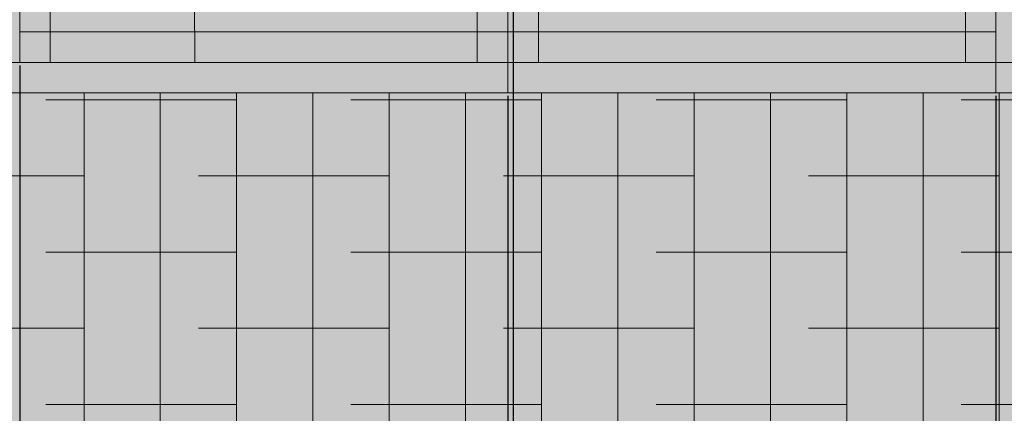
# Model space of a CAD drawing. Units: millimetres. Extents: x 11032 to 26788, y 3406 to 24505.
# Tile 13 of 78: x 17145 to 18758, y 6736 to 7381. Entities that reach past the tile are written whole.
import ezdxf

# ---------------------------------------------------------------- set-up
doc = ezdxf.new("R2010")
doc.units = ezdxf.units.MM
doc.header["$MEASUREMENT"] = 0
for name, color, linetype, lineweight in [('A-ANNO-DIMS', 2, 'Continuous', 18), ('A-GLAZ', 250, 'Continuous', 20), ('A-WALL-INTR', 8, 'Continuous', 18), ('A-WALL-PLIN-PATT', 253, 'Continuous', 13)]:
    doc.layers.add(name, color=color, linetype=linetype, lineweight=lineweight)
doc.layers.add('A-GLAZ-FRAM-PATT', color=250, linetype='Continuous', lineweight=13, true_color=0x262627)
doc.layers.add('A-WALL-INTR-PATT', color=251, linetype='Continuous', lineweight=13, true_color=0x6c6b6a)
doc.styles.get("Standard").update_dxf_attribs({"font": 'arial.ttf'})
doc.dimstyles.get("Standard").update_dxf_attribs({"dimtxt": 150, "dimasz": 100, "dimexe": 10, "dimexo": 5, "dimgap": 5, "dimtad": 0, "dimtih": 1, "dimtoh": 1, "dimdec": 0, "dimzin": 0, "dimdsep": 46, "dimtxsty": 'Standard', "dimcen": 0.09, "dimadec": 0, "dimazin": 0, "dimtfac": 1, "dimtdec": 0, "dimtofl": 0, "dimtmove": 0, "dimatfit": 3, "dimfxl": 1, "dimtolj": 1, "dimtzin": 0, "dimarcsym": 0})

# ---------------------------------------------------------------- blocks, each defined once
blk = doc.blocks.new('*D36')
at = {"layer": 'A-ANNO-DIMS', "color": 0, "lineweight": -2, "transparency": 16777216}
for p, q in [((12301.3, 17115.9), (12301.3, 24416.9)), ((25397.4, 4466.4), (25397.4, 24416.9)), ((12401.3, 24406.9), (18569.2, 24406.9)), ((25297.4, 24406.9), (19129.5, 24406.9))]:
    blk.add_line(p, q, dxfattribs=at)
at = {"layer": 'A-ANNO-DIMS', "color": 0, "transparency": 16777216}
for points in [[(12401.3, 24423.5), (12401.3, 24390.2), (12301.3, 24406.9)], [(25297.4, 24423.5), (25297.4, 24390.2), (25397.4, 24406.9)]]:
    blk.add_solid(points, dxfattribs=at)
at = {"layer": 'Defpoints', "color": 0, "transparency": 16777216}
for p in [(25397.4, 24406.9), (12301.3, 17110.9), (25397.4, 4461.4)]:
    blk.add_point(p, dxfattribs=at)
at = {"layer": 'A-ANNO-DIMS', "color": 0, "transparency": 16777216, "insert": (18849.3, 24406.9), "char_height": 150, "attachment_point": 5}
blk.add_mtext('\\A1;13096', dxfattribs=at)
blk = doc.blocks.new('*D37')
at = {"layer": 'A-ANNO-DIMS', "color": 0, "lineweight": -2, "transparency": 16777216}
for p, q in [((18087.7, 23450.4), (11334.8, 23450.4)), ((11344.8, 23350.4), (11344.8, 14037.5)), ((11344.8, 4561.4), (11344.8, 13874.3)), ((12927.7, 4461.4), (11334.8, 4461.4))]:
    blk.add_line(p, q, dxfattribs=at)
at = {"layer": 'A-ANNO-DIMS', "color": 0, "transparency": 16777216}
for points in [[(11328.1, 23350.4), (11361.4, 23350.4), (11344.8, 23450.4)], [(11328.1, 4561.4), (11361.4, 4561.4), (11344.8, 4461.4)]]:
    blk.add_solid(points, dxfattribs=at)
at = {"layer": 'Defpoints', "color": 0, "transparency": 16777216}
for p in [(11344.8, 23450.4), (18092.7, 23450.4), (12932.7, 4461.4)]:
    blk.add_point(p, dxfattribs=at)
at = {"layer": 'A-ANNO-DIMS', "color": 0, "transparency": 16777216, "insert": (11344.8, 13955.9), "char_height": 150, "attachment_point": 5}
blk.add_mtext('\\A1;18989', dxfattribs=at)
blk = doc.blocks.new('*D49')
at = {"layer": 'A-ANNO-DIMS', "color": 0, "lineweight": -2, "transparency": 16777216}
for p, q in [((17953.5, 10206.4), (17953.5, 3494.9)), ((14996.4, 6406.4), (14996.4, 3494.9)), ((15096.4, 3504.9), (16244.7, 3504.9)), ((17853.5, 3504.9), (16705.2, 3504.9))]:
    blk.add_line(p, q, dxfattribs=at)
at = {"layer": 'A-ANNO-DIMS', "color": 0, "transparency": 16777216}
for points in [[(15096.4, 3521.6), (15096.4, 3488.2), (14996.4, 3504.9)], [(17853.5, 3521.6), (17853.5, 3488.2), (17953.5, 3504.9)]]:
    blk.add_solid(points, dxfattribs=at)
at = {"layer": 'Defpoints', "color": 0, "transparency": 16777216}
for p in [(17953.5, 10211.4), (14996.4, 6411.4), (17953.5, 3504.9)]:
    blk.add_point(p, dxfattribs=at)
at = {"layer": 'A-ANNO-DIMS', "color": 0, "transparency": 16777216, "insert": (16474.9, 3504.9), "char_height": 150, "attachment_point": 5}
blk.add_mtext('\\A1;2957', dxfattribs=at)
blk = doc.blocks.new('*D50')
at = {"layer": 'A-ANNO-DIMS', "color": 0, "lineweight": -2, "transparency": 16777216}
for p, q in [((19697.4, 16000.7), (19697.4, 3494.9)), ((17953.5, 10206.4), (17953.5, 3494.9)), ((18053.5, 3504.9), (18603.8, 3504.9)), ((19597.4, 3504.9), (19047, 3504.9))]:
    blk.add_line(p, q, dxfattribs=at)
at = {"layer": 'A-ANNO-DIMS', "color": 0, "transparency": 16777216}
for points in [[(18053.5, 3521.6), (18053.5, 3488.2), (17953.5, 3504.9)], [(19597.4, 3521.6), (19597.4, 3488.2), (19697.4, 3504.9)]]:
    blk.add_solid(points, dxfattribs=at)
at = {"layer": 'Defpoints', "color": 0, "transparency": 16777216}
for p in [(19697.4, 16005.7), (17953.5, 10211.4), (19697.4, 3504.9)]:
    blk.add_point(p, dxfattribs=at)
at = {"layer": 'A-ANNO-DIMS', "color": 0, "transparency": 16777216, "insert": (18825.4, 3504.9), "char_height": 150, "attachment_point": 5}
blk.add_mtext('\\A1;1744', dxfattribs=at)
blk = doc.blocks.new('*D57')
at = {"layer": 'A-ANNO-DIMS', "color": 0, "lineweight": -2, "transparency": 16777216}
for p, q in [((14994.7, 7266.4), (14994.7, 24416.9)), ((20894.7, 7266.4), (20894.7, 24416.9)), ((15094.7, 24406.9), (17716, 24406.9)), ((20794.7, 24406.9), (18173.4, 24406.9))]:
    blk.add_line(p, q, dxfattribs=at)
at = {"layer": 'A-ANNO-DIMS', "color": 0, "transparency": 16777216}
for points in [[(15094.7, 24423.5), (15094.7, 24390.2), (14994.7, 24406.9)], [(20794.7, 24423.5), (20794.7, 24390.2), (20894.7, 24406.9)]]:
    blk.add_solid(points, dxfattribs=at)
at = {"layer": 'Defpoints', "color": 0, "transparency": 16777216}
for p in [(20894.7, 24406.9), (14994.7, 7261.4), (20894.7, 7261.4)]:
    blk.add_point(p, dxfattribs=at)
at = {"layer": 'A-ANNO-DIMS', "color": 0, "transparency": 16777216, "insert": (17944.7, 24406.9), "char_height": 150, "attachment_point": 5}
blk.add_mtext('\\A1;5900', dxfattribs=at)
blk = doc.blocks.new('*D62')
at = {"layer": 'A-ANNO-DIMS', "color": 0, "lineweight": -2, "transparency": 16777216}
for p, q in [((17144.7, 7306.4), (17144.7, 3494.9)), ((17944.7, 7256.4), (17944.7, 3494.9)), ((17244.7, 3504.9), (17374.2, 3504.9)), ((17844.7, 3504.9), (17715.3, 3504.9))]:
    blk.add_line(p, q, dxfattribs=at)
at = {"layer": 'A-ANNO-DIMS', "color": 0, "transparency": 16777216}
for points in [[(17244.7, 3521.6), (17244.7, 3488.2), (17144.7, 3504.9)], [(17844.7, 3521.6), (17844.7, 3488.2), (17944.7, 3504.9)]]:
    blk.add_solid(points, dxfattribs=at)
at = {"layer": 'Defpoints', "color": 0, "transparency": 16777216}
for p in [(17144.7, 7311.4), (17944.7, 7261.4), (17944.7, 3504.9)]:
    blk.add_point(p, dxfattribs=at)
at = {"layer": 'A-ANNO-DIMS', "color": 0, "transparency": 16777216, "insert": (17544.7, 3504.9), "char_height": 150, "attachment_point": 5}
blk.add_mtext('\\A1;800', dxfattribs=at)
blk = doc.blocks.new('*D63')
at = {"layer": 'A-ANNO-DIMS', "color": 0, "lineweight": -2, "transparency": 16777216}
for p, q in [((17944.7, 7256.4), (17944.7, 3494.9)), ((18744.7, 7256.4), (18744.7, 3494.9)), ((18044.7, 3504.9), (18174.2, 3504.9)), ((18644.7, 3504.9), (18515.3, 3504.9))]:
    blk.add_line(p, q, dxfattribs=at)
at = {"layer": 'A-ANNO-DIMS', "color": 0, "transparency": 16777216}
for points in [[(18044.7, 3521.6), (18044.7, 3488.2), (17944.7, 3504.9)], [(18644.7, 3521.6), (18644.7, 3488.2), (18744.7, 3504.9)]]:
    blk.add_solid(points, dxfattribs=at)
at = {"layer": 'Defpoints', "color": 0, "transparency": 16777216}
for p in [(17944.7, 7261.4), (18744.7, 7261.4), (18744.7, 3504.9)]:
    blk.add_point(p, dxfattribs=at)
at = {"layer": 'A-ANNO-DIMS', "color": 0, "transparency": 16777216, "insert": (18344.7, 3504.9), "char_height": 150, "attachment_point": 5}
blk.add_mtext('\\A1;800', dxfattribs=at)
blk = doc.blocks.new('*D64')
at = {"layer": 'A-ANNO-DIMS', "color": 0, "lineweight": -2, "transparency": 16777216}
for p, q in [((18744.7, 7256.4), (18744.7, 3494.9)), ((19544.7, 7256.4), (19544.7, 3494.9)), ((18844.7, 3504.9), (18974.2, 3504.9)), ((19444.7, 3504.9), (19315.3, 3504.9))]:
    blk.add_line(p, q, dxfattribs=at)
at = {"layer": 'A-ANNO-DIMS', "color": 0, "transparency": 16777216}
for points in [[(18844.7, 3521.6), (18844.7, 3488.2), (18744.7, 3504.9)], [(19444.7, 3521.6), (19444.7, 3488.2), (19544.7, 3504.9)]]:
    blk.add_solid(points, dxfattribs=at)
at = {"layer": 'Defpoints', "color": 0, "transparency": 16777216}
for p in [(18744.7, 7261.4), (19544.7, 7261.4), (19544.7, 3504.9)]:
    blk.add_point(p, dxfattribs=at)
at = {"layer": 'A-ANNO-DIMS', "color": 0, "transparency": 16777216, "insert": (19144.7, 3504.9), "char_height": 150, "attachment_point": 5}
blk.add_mtext('\\A1;800', dxfattribs=at)
blk = doc.blocks.new('*D66')
at = {"layer": 'A-ANNO-DIMS', "color": 0, "lineweight": -2, "transparency": 16777216}
for p, q in [((16725.9, 10296), (16725.9, 3494.9)), ((19150.9, 10296), (19150.9, 3494.9)), ((16825.9, 3504.9), (17707.6, 3504.9)), ((19050.9, 3504.9), (18169.3, 3504.9))]:
    blk.add_line(p, q, dxfattribs=at)
at = {"layer": 'A-ANNO-DIMS', "color": 0, "transparency": 16777216}
for points in [[(16825.9, 3521.6), (16825.9, 3488.2), (16725.9, 3504.9)], [(19050.9, 3521.6), (19050.9, 3488.2), (19150.9, 3504.9)]]:
    blk.add_solid(points, dxfattribs=at)
at = {"layer": 'Defpoints', "color": 0, "transparency": 16777216}
for p in [(16725.9, 10301), (19150.9, 10301), (19150.9, 3504.9)]:
    blk.add_point(p, dxfattribs=at)
at = {"layer": 'A-ANNO-DIMS', "color": 0, "transparency": 16777216, "insert": (17938.4, 3504.9), "char_height": 150, "attachment_point": 5}
blk.add_mtext('\\A1;2425', dxfattribs=at)
blk = doc.blocks.new('*D69')
at = {"layer": 'A-ANNO-DIMS', "color": 0, "lineweight": -2, "transparency": 16777216}
for p, q in [((13957, 9938), (14057, 9938)), ((14057, 9938), (15432.5, 8991)), ((17944.6, 7261.4), (17944.8, 7261.4)), ((17944.7, 7261.3), (17944.7, 7261.5))]:
    blk.add_line(p, q, dxfattribs=at)
at = {"layer": 'A-ANNO-DIMS', "color": 0, "transparency": 16777216}
blk.add_solid([(15442, 9004.7), (15423.1, 8977.2), (15514.9, 8934.2)], dxfattribs=at)
at = {"layer": 'Defpoints', "color": 0, "transparency": 16777216}
for p in [(15514.9, 8934.2), (17944.7, 7261.4)]:
    blk.add_point(p, dxfattribs=at)
at = {"layer": 'A-ANNO-DIMS', "color": 0, "transparency": 16777216, "insert": (13494, 9938), "char_height": 150, "attachment_point": 5}
blk.add_mtext('\\A1;2X R2950', dxfattribs=at)
blk = doc.blocks.new('*D70')
at = {"layer": 'A-ANNO-DIMS', "color": 0, "lineweight": -2, "transparency": 16777216}
for p, q in [((18044.7, 11901.4), (17944.7, 11901.4)), ((17944.7, 11901.4), (17944.7, 10261.4)), ((17944.6, 7261.4), (17944.8, 7261.4)), ((17944.7, 7261.3), (17944.7, 7261.5))]:
    blk.add_line(p, q, dxfattribs=at)
at = {"layer": 'A-ANNO-DIMS', "color": 0, "transparency": 16777216}
blk.add_solid([(17928, 10261.4), (17961.4, 10261.4), (17944.7, 10161.4)], dxfattribs=at)
at = {"layer": 'Defpoints', "color": 0, "transparency": 16777216}
for p in [(17944.7, 10161.4), (17944.7, 7261.4)]:
    blk.add_point(p, dxfattribs=at)
at = {"layer": 'A-ANNO-DIMS', "color": 0, "transparency": 16777216, "insert": (18345.2, 11901.4), "char_height": 150, "attachment_point": 5}
blk.add_mtext('\\A1;R2900', dxfattribs=at)

msp = doc.modelspace()

# ---------------------------------------------------------------- hatches: boundary and pattern name
at = {"layer": 'A-GLAZ-FRAM-PATT'}
h = msp.add_hatch(color=256, dxfattribs=at)
h.paths.add_polyline_path([(17944.704, 7311.399), (16344.704, 7311.399), (16344.704, 7261.399), (17944.704, 7261.399)], flags=17)
h.paths.add_polyline_path([(16344.704, 7311.399), (15045.135, 7311.399, -0.98290472), (20844.273, 7311.399), (19544.704, 7311.399), (19544.704, 7261.399), (20894.704, 7261.399, 0.51484406), (16985.951, 10051.255, 0.32026791), (14994.704, 7261.399), (16344.704, 7261.399)])
h.paths.add_polyline_path([(18744.704, 7311.399), (17944.704, 7311.399), (17944.704, 7261.399), (18744.704, 7261.399)], flags=17)
h.paths.add_polyline_path([(19544.704, 7311.399), (18744.704, 7311.399), (18744.704, 7261.399), (19544.704, 7261.399)], flags=17)
h.paths.add_polyline_path([(18694.704, 7361.399), (17994.704, 7361.399), (17994.704, 7311.399), (18694.704, 7311.399)], flags=17)
h.paths.add_polyline_path([(18744.704, 7361.399), (18694.704, 7361.399), (18694.704, 7311.399), (18744.704, 7311.399)], flags=17)
h.paths.add_polyline_path([(17194.704, 7361.399), (17144.704, 7361.399), (17144.704, 7311.399), (17194.704, 7311.399)], flags=17)
h.paths.add_polyline_path([(17431.432, 7361.399), (17194.704, 7361.399), (17194.704, 7311.399), (17431.699, 7311.399)], flags=17)
h.paths.add_polyline_path([(17894.704, 7361.399), (17431.432, 7361.399), (17431.699, 7311.399), (17894.704, 7311.399)], flags=17)
h.paths.add_polyline_path([(17944.704, 7361.399), (17894.704, 7361.399), (17894.704, 7311.399), (17944.704, 7311.399)], flags=17)
h.paths.add_polyline_path([(17994.704, 7361.399), (17944.704, 7361.399), (17944.704, 7311.399), (17994.704, 7311.399)], flags=17)
h = msp.add_hatch(color=256, dxfattribs=at)
h.paths.add_polyline_path([(16734.609, 9896.863, 0.03337538), (16394.704, 9712.419), (16394.704, 7804.617), (16431.407, 7804.617), (16458.237, 7920.19), (16398.691, 8130.481), (16448.141, 8186.871), (16512.813, 8185.465, -0.15483335), (16566.508, 7929.387, -0.14766935), (16637.008, 7933.112), (16627.369, 7874.366), (16647.499, 7804.617), (16742.939, 7804.617)])
h.paths.add_polyline_path([(17094.704, 9961.399), (16886.403, 9961.399, 0.01422214), (16734.609, 9896.863), (16741.107, 8264.696), (17094.704, 8264.696)])
h.paths.add_polyline_path([(17417.202, 10027.292), (17194.704, 10011.399), (17194.704, 8264.696), (17426.61, 8264.696)])
h.paths.add_polyline_path([(17144.704, 8239.696), (17094.704, 8239.696), (17094.704, 7361.399), (16394.704, 7361.399), (16394.704, 7493.572), (16379.987, 7430.181), (16369.733, 7430.232), (16394.704, 7537.793), (16394.704, 7559.524), (16359.112, 7561.363), (16344.704, 7499.3), (16344.704, 7311.399), (17144.704, 7311.399)])
h.paths.add_polyline_path([(17194.704, 8239.696), (17144.704, 8239.696), (17144.704, 7361.399), (17194.704, 7361.399)])
h = msp.add_hatch(color=256, dxfattribs=at)
h.paths.add_polyline_path([(17944.704, 8239.696), (17894.704, 8239.696), (17894.704, 7796.661), (17944.704, 7796.661)])
h.paths.add_polyline_path([(17994.704, 8239.696), (17944.704, 8239.696), (17944.704, 7796.661), (17994.704, 7796.661)])
h.paths.add_polyline_path([(17944.704, 7785.559), (17894.704, 7785.559), (17894.704, 7361.399), (17944.704, 7361.399)])
h.paths.add_polyline_path([(17994.704, 7785.559), (17944.704, 7785.559), (17944.704, 7361.399), (17994.704, 7361.399)])
h.paths.add_polyline_path([(18744.704, 8239.696), (18694.704, 8239.696), (18694.704, 7361.399), (18744.704, 7361.399)])
h.paths.add_polyline_path([(18794.704, 8239.696), (18744.704, 8239.696), (18744.704, 7311.399), (19544.704, 7311.399), (19544.704, 7613.382), (19531.043, 7566.052), (19520.62, 7566), (19544.704, 7649.444), (19544.704, 7691.272), (19514.696, 7689.722), (19494.704, 7620.453), (19494.704, 7361.399), (18794.704, 7361.399)])
at = {"layer": 'A-WALL-INTR-PATT'}
h = msp.add_hatch(color=256, dxfattribs=at)
h.set_gradient(color1=(254, 234, 185), color2=(254, 204, 102), name='CURVED')
h.paths.add_polyline_path([(15260.167, 7582.928), (15062.56, 7582.722, 0.02345098), (15045.135, 7311.399), (15314.374, 7311.399)])
h.paths.add_polyline_path([(15413.095, 7583.087), (15260.167, 7582.928), (15314.374, 7311.399), (15467.334, 7311.399)])
h.paths.add_polyline_path([(15531.986, 7554.365), (15523.82, 7583.203), (15413.095, 7583.087), (15467.334, 7311.399), (15790.119, 7311.399), (15790.667, 7566.433), (15785.748, 7583.476), (15718.988, 7583.406), (15701.389, 7507.6), (15736.743, 7385.107), (15726.32, 7385.159), (15696.749, 7487.614), (15695.471, 7482.107), (15685.217, 7482.158), (15691.06, 7507.327), (15690.552, 7509.088), (15650.881, 7511.137), (15649.743, 7506.234), (15684.627, 7385.366), (15674.204, 7385.418), (15646.227, 7482.352), (15633.946, 7482.413), (15639.413, 7505.961), (15637.723, 7511.817), (15584.344, 7514.575), (15554.498, 7386.013), (15544.244, 7386.064), (15574.2, 7515.099), (15533.623, 7517.195), (15503.228, 7386.268), (15492.974, 7386.319)])
h.paths.add_polyline_path([(16344.704, 7499.3), (16328.717, 7430.435), (16318.463, 7430.486), (16344.704, 7543.521), (16344.704, 7584.059), (16080.595, 7583.783), (16085.615, 7566.39), (16075.192, 7566.442), (16070.19, 7583.773), (16028.57, 7583.729), (16033.5, 7566.649), (16023.077, 7566.701), (16018.165, 7583.718), (15907.156, 7583.603), (15903.371, 7567.296), (15893.116, 7567.347), (15896.888, 7583.592), (15855.814, 7583.549), (15852.409, 7568.882), (15877.716, 7481.201), (15867.293, 7481.253), (15844.553, 7560.041), (15844.691, 7311.399), (16344.704, 7311.399)])
h.paths.add_polyline_path([(15844.553, 7560.041), (15842.372, 7567.599), (15841.846, 7567.602), (15842.08, 7568.609), (15837.773, 7583.53), (15796.153, 7583.487), (15825.6, 7481.46), (15815.177, 7481.512), (15790.667, 7566.433), (15790.119, 7311.399), (15844.691, 7311.399)])
h.paths.add_polyline_path([(16394.704, 7493.572), (16379.987, 7430.181), (16369.733, 7430.232), (16394.704, 7537.793), (16394.704, 7559.524), (16359.112, 7561.363), (16344.704, 7499.3), (16344.704, 7311.399), (17144.704, 7311.399), (17144.704, 7584.893), (17094.704, 7584.841), (17094.704, 7361.399), (16394.704, 7361.399)])
h.paths.add_polyline_path([(17430.237, 7585.191), (17194.704, 7584.945), (17194.704, 7361.399), (17431.432, 7361.399)])
h.paths.add_polyline_path([(17894.704, 7585.675), (17748.458, 7585.522), (17754.673, 7563.99), (17744.25, 7564.042), (17738.053, 7585.511), (17696.433, 7585.468), (17702.557, 7564.249), (17692.134, 7564.301), (17686.028, 7585.457), (17577.175, 7585.344), (17572.428, 7564.896), (17562.174, 7564.947), (17566.907, 7585.333), (17525.833, 7585.29), (17521.158, 7565.151), (17510.903, 7565.202), (17515.565, 7585.28), (17430.237, 7585.191), (17431.432, 7361.399), (17894.704, 7361.399)])
h.paths.add_polyline_path([(18694.704, 7586.509), (18404.857, 7586.207), (18425.604, 7496.839), (18415.35, 7496.788), (18394.593, 7586.196), (18353.54, 7586.153), (18374.333, 7496.584), (18364.079, 7496.533), (18343.276, 7586.142), (18270.386, 7586.066), (18244.373, 7495.938), (18233.95, 7495.887), (18259.974, 7586.056), (18218.329, 7586.012), (18192.257, 7495.679), (18181.834, 7495.628), (18207.918, 7586.001), (17994.704, 7585.779), (17994.704, 7361.399), (18694.704, 7361.399)])
h.paths.add_polyline_path([(19317.979, 7532.562), (19264.6, 7535.319), (19234.754, 7406.757), (19224.5, 7406.808), (19254.456, 7535.844), (19213.879, 7537.94), (19183.484, 7407.012), (19173.23, 7407.063), (19212.242, 7575.11), (19208.862, 7587.045), (19127.433, 7586.96), (19124.467, 7576.487), (19163.48, 7408.44), (19153.225, 7408.389), (19122.83, 7539.317), (19082.253, 7537.22), (19112.209, 7408.185), (19101.955, 7408.134), (19072.109, 7536.696), (19035.898, 7534.825), (19044.517, 7497.701), (19034.262, 7497.65), (19025.754, 7534.301), (19018.73, 7533.938), (18982.249, 7407.539), (18971.826, 7407.487), (19008.164, 7533.392), (18985.177, 7532.205), (18993.246, 7497.447), (18982.992, 7497.396), (18975.033, 7531.681), (18965.902, 7531.209), (18930.133, 7407.28), (18919.71, 7407.228), (18955.336, 7530.663), (18946.129, 7586.771), (18889.236, 7586.712), (18863.286, 7496.801), (18852.863, 7496.749), (18878.825, 7586.701), (18837.179, 7586.657), (18811.17, 7496.542), (18800.747, 7496.49), (18826.768, 7586.647), (18794.704, 7586.613), (18794.704, 7361.399), (19494.704, 7361.399), (19494.704, 7587.343), (19485.145, 7587.333), (19478.928, 7565.793), (19468.505, 7565.741), (19473, 7581.318), (19466.812, 7581.349), (19465.091, 7587.312), (19423.471, 7587.269), (19425.12, 7581.556), (19414.696, 7581.608), (19413.066, 7587.258), (19390.882, 7587.235), (19381.373, 7529.286), (19416.999, 7405.852), (19406.576, 7405.903), (19370.808, 7529.832), (19328.545, 7532.016), (19364.883, 7406.111), (19354.46, 7406.162)])
h.paths.add_polyline_path([(19990.261, 7587.86), (19974.192, 7587.843), (19950.141, 7504.512), (19939.718, 7504.46), (19963.781, 7587.832), (19883.217, 7587.748), (19899.552, 7517.385), (19889.298, 7517.334), (19872.954, 7587.737), (19831.9, 7587.695), (19848.282, 7517.13), (19838.028, 7517.079), (19821.637, 7587.684), (19738.846, 7587.598), (19718.322, 7516.484), (19707.899, 7516.432), (19728.435, 7587.587), (19707.489, 7587.565), (19712.274, 7566.953), (19702.02, 7566.902), (19697.225, 7587.554), (19686.79, 7587.543), (19666.206, 7516.225), (19655.783, 7516.173), (19676.379, 7587.532), (19656.172, 7587.511), (19661.003, 7566.698), (19650.749, 7566.647), (19645.908, 7587.501), (19544.704, 7587.395), (19544.704, 7311.399), (19990.261, 7311.399)])
h.paths.add_polyline_path([(20190.261, 7455.206), (20179.112, 7455.151), (20190.261, 7493.779), (20190.261, 7579.754), (20173.188, 7578.872), (20169.478, 7566.018), (20183.488, 7505.671), (20173.234, 7505.62), (20163.789, 7546.305), (20137.42, 7454.943), (20126.997, 7454.892), (20159.149, 7566.291), (20154.102, 7588.03), (20113.048, 7587.988), (20132.217, 7505.417), (20121.963, 7505.366), (20102.785, 7587.977), (20026.249, 7587.897), (20002.257, 7504.771), (19990.261, 7504.711), (19990.261, 7311.399), (20190.261, 7311.399)])
h.paths.add_polyline_path([(20340.261, 7543.283), (20330.117, 7586.98), (20289.54, 7584.884), (20319.496, 7455.848), (20309.241, 7455.797), (20279.396, 7584.359), (20226.017, 7581.602), (20190.261, 7457.717), (20190.261, 7311.399), (20340.261, 7311.399)])
h.paths.add_polyline_path([(20826.171, 7588.731), (20340.261, 7588.225), (20340.261, 7587.504), (20370.766, 7456.103), (20360.512, 7456.052), (20340.261, 7543.283), (20340.261, 7311.399), (20844.273, 7311.399, 0.02397257)])
at = {"layer": 'A-WALL-PLIN-PATT'}
h = msp.add_hatch(color=256, dxfattribs=at)
h.set_gradient(color1=(99, 100, 102), color2=(199, 200, 202), name='CYLINDER')
edge = h.paths.add_edge_path()
edge.add_arc((17944.704, 7261.399), 2950, 180, 181.942602)
edge.add_line((14996.399, 7161.399), (12932.665, 7161.399))
edge.add_line((12932.665, 7161.399), (12932.665, 6411.399))
edge.add_line((12932.665, 6411.399), (25397.404, 6411.399))
edge.add_line((25397.404, 6411.399), (25397.404, 7161.399))
edge.add_line((25397.404, 7161.399), (22955.171, 7161.399))
edge.add_spline(control_points=[(22955.171, 7161.399), (22875.95, 7159.113), (22796.729, 7156.828), (22718.347, 7161.399)], knot_values=[0, 0, 0, 0, 236.62389499, 236.62389499, 236.62389499, 236.62389499], degree=3, periodic=0)
edge.add_spline(control_points=[(22718.347, 7161.399), (22709.27, 7161.929), (22517.84, 7175.049), (22332.009, 7233.921), (22155.123, 7291.176)], knot_values=[236.62389499, 236.62389499, 236.62389499, 236.62389499, 264.02785008, 815.24414583, 815.24414583, 815.24414583, 815.24414583], degree=3, periodic=0)
edge.add_line((22155.123, 7291.176), (22155.123, 7161.399))
edge.add_line((22155.123, 7161.399), (20893.008, 7161.399))
edge.add_arc((17944.704, 7261.399), 2950, 358.057398, 360)
edge.add_line((20894.704, 7261.399), (14994.704, 7261.399))
h.paths.add_polyline_path([(14996.399, 6261.399), (14822.389, 6162.807), (21067.019, 6162.807), (20893.008, 6261.399)])
h.paths.add_polyline_path([(14822.224, 6012.807), (14648.718, 5913.331), (21240.69, 5913.331), (21067.183, 6012.807)])
h.paths.add_polyline_path([(21414.634, 5661.399), (21414.635, 5662.395), (21241.977, 5763.336), (14647.43, 5763.336), (14474.772, 5662.395), (14474.774, 5661.399)])
h.paths.add_polyline_path([(14474.964, 5512.395), (14302.433, 5411.236), (21586.974, 5411.236), (21414.443, 5512.395)])
h.paths.add_polyline_path([(14301.435, 5261.24), (14128.313, 5161.097), (21761.094, 5161.097), (21587.972, 5261.24)])
h.paths.add_polyline_path([(22722.526, 4461.399), (21760.979, 5011.097), (14128.428, 5011.097), (13166.882, 4461.399)])
h = msp.add_hatch(dxfattribs=at)
h.set_pattern_fill('ANSI38', color=256, scale=1000, angle=45, style=0)
edge = h.paths.add_edge_path()
edge.add_line((25397.404, 6411.399), (25397.404, 7161.399))
edge.add_line((25397.404, 7161.399), (22955.171, 7161.399))
edge.add_spline(control_points=[(22955.171, 7161.399), (22875.95, 7159.113), (22796.729, 7156.828), (22718.347, 7161.399)], knot_values=[0, 0, 0, 0, 236.62389499, 236.62389499, 236.62389499, 236.62389499], degree=3, periodic=0)
edge.add_spline(control_points=[(22718.347, 7161.399), (22709.27, 7161.929), (22517.84, 7175.049), (22332.009, 7233.921), (22155.123, 7291.176)], knot_values=[236.62389499, 236.62389499, 236.62389499, 236.62389499, 264.02785008, 815.24414583, 815.24414583, 815.24414583, 815.24414583], degree=3, periodic=0)
edge.add_line((22155.123, 7291.176), (22155.123, 7161.399))
edge.add_line((22155.123, 7161.399), (20893.008, 7161.399))
edge.add_arc((17944.704, 7261.399), 2950, 358.057398, 360)
edge.add_line((20894.704, 7261.399), (14994.704, 7261.399))
edge.add_arc((17944.704, 7261.399), 2950, 180, 181.942602)
edge.add_line((14996.399, 7161.399), (12932.665, 7161.399))
edge.add_line((12932.665, 7161.399), (12932.665, 6411.399))
edge.add_line((12932.665, 6411.399), (25397.404, 6411.399))

# ---------------------------------------------------------------- linework, layer by layer
at = {"layer": 'A-GLAZ'}
for p, q in [((17944.704, 7261.399), (17944.704, 10161.399)), ((17894.704, 7311.399), (17894.704, 10061.399)), ((17994.704, 7311.399), (17994.704, 10061.399)), ((17144.704, 7311.399), (17144.704, 10048.871)), ((18744.704, 7261.399), (18744.704, 10048.871)), ((17194.704, 7311.399), (17194.704, 10011.399)), ((18694.704, 7311.399), (18694.704, 10011.399)), ((17144.704, 7361.399), (17944.704, 7361.399)), ((17944.704, 7361.399), (18744.704, 7361.399)), ((15045.135, 7311.399), (20844.273, 7311.399)), ((14994.704, 7261.399), (20894.704, 7261.399))]:
    msp.add_line(p, q, dxfattribs=at)
for radius, start, end in [(2950, 358.057398, 108.965621), (2900, 0.987907, 179.012093)]:
    msp.add_arc((17944.704, 7261.399), radius, start, end, dxfattribs=at)
at = {"layer": 'A-WALL-INTR'}
msp.add_line((17431.699, 7311.399), (17417.202, 10027.292), dxfattribs=at)

# ---------------------------------------------------------------- dimensions: what is measured, and where the dimension line sits
at = {"layer": 'A-ANNO-DIMS'}
for base, p1, p2, picture, middle in [((25397.404, 24406.858), (12301.265, 17110.885), (25397.404, 4461.399), '*D36', (18849.334, 24406.858)), ((20894.704, 24406.858), (14994.704, 7261.399), (20894.704, 7261.399), '*D57', (17944.704, 24406.858)), ((19697.404, 3504.899), (17953.455, 10211.41), (19697.404, 16005.71), '*D50', (18825.429, 3504.899)), ((19150.949, 3504.899), (16725.949, 10301.016), (19150.949, 10301.016), '*D66', (17938.449, 3504.899)), ((17953.455, 3504.899), (14996.399, 6411.399), (17953.455, 10211.41), '*D49', (16474.927, 3504.899)), ((17944.704, 3504.899), (17144.704, 7311.399), (17944.704, 7261.399), '*D62', (17544.704, 3504.899)), ((18744.704, 3504.899), (17944.704, 7261.399), (18744.704, 7261.399), '*D63', (18344.704, 3504.899)), ((19544.704, 3504.899), (18744.704, 7261.399), (19544.704, 7261.399), '*D64', (19144.704, 3504.899))]:
    dim = msp.add_linear_dim(base=base, p1=p1, p2=p2, dimstyle='Standard', override={"dimdec": 0, "dimlfac": 1, "dimrnd": 0, "dimzin": 0, "dimdsep": 46, "dimlunit": 2}, dxfattribs=at)
    dim.commit()
    dim.dimension.update_dxf_attribs({"geometry": picture, "text_midpoint": middle})
dim = msp.add_linear_dim(base=(11344.765, 23450.358), p1=(12932.665, 4461.399), p2=(18092.739, 23450.358), angle=90, dimstyle='Standard', override={"dimdec": 0, "dimlfac": 1, "dimrnd": 0, "dimzin": 0, "dimdsep": 46, "dimlunit": 2}, dxfattribs=at)
dim.commit()
dim.dimension.update_dxf_attribs({"geometry": '*D37', "text_midpoint": (11344.765, 13955.879)})
dim = msp.add_radius_dim(center=(17944.704, 7261.399), mpoint=(17944.704, 10161.399), dimstyle='Standard', override={"dimdec": 0, "dimlfac": 1, "dimrnd": 0, "dimzin": 0, "dimdsep": 46, "dimlunit": 2}, dxfattribs=at)
dim.commit()
dim.dimension.update_dxf_attribs({"geometry": '*D70', "text_midpoint": (18345.202, 11901.399), "dimtype": 164})
dim = msp.add_radius_dim(center=(17944.704, 7261.399), mpoint=(15514.87, 8934.244), text='2X <>', dimstyle='Standard', override={"dimdec": 0, "dimlfac": 1, "dimrnd": 0, "dimzin": 0, "dimdsep": 46, "dimlunit": 2}, dxfattribs=at)
dim.commit()
dim.dimension.update_dxf_attribs({"geometry": '*D69', "text_midpoint": (13494.04, 9937.951), "dimtype": 164})

doc.saveas('drawing.dxf')
